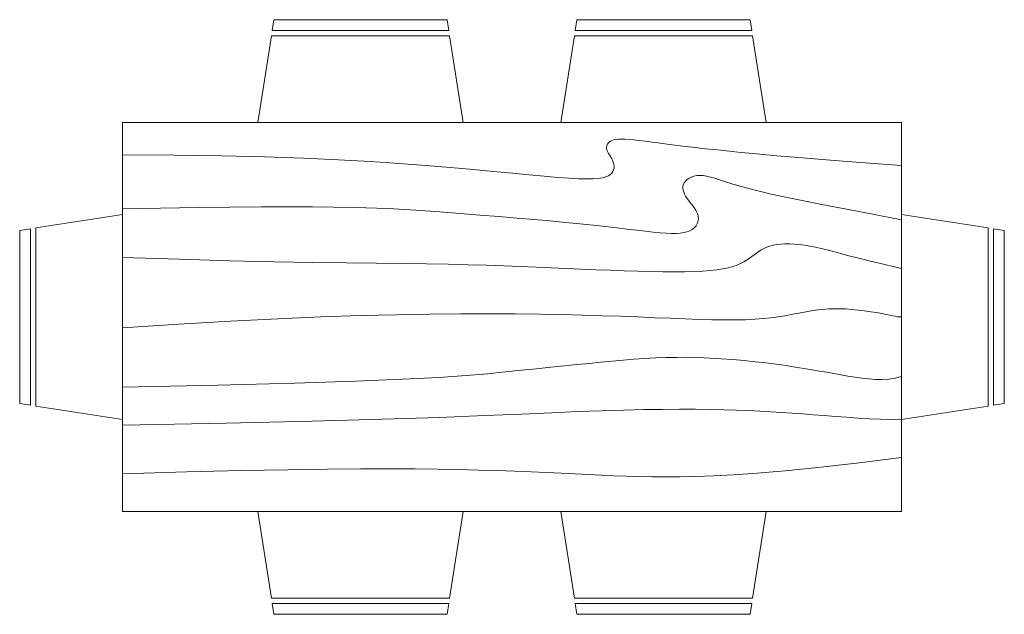
# Model space of a CAD drawing. Units: inches. Extents: x 2208 to 4689, y 1219 to 3512.
# Tile 5 of 5: x 4598 to 4689, y 3457 to 3512. Entities that reach past the tile are written whole.
import ezdxf

# ---------------------------------------------------------------- set-up
doc = ezdxf.new("R2010")
doc.units = ezdxf.units.IN
doc.layers.add('A-FURN', color=8, linetype='Continuous', lineweight=18)

# ---------------------------------------------------------------- blocks, each defined once
blk = doc.blocks.new('Dining Set - 36 x 72 in.')
for p, q in [((-22, 27.5), (-22.1562, 26.50042)), ((-22, 27.5), (-6, 27.5)), ((-5.8437, 26.49966), (-6, 27.5)), ((6, 27.5), (5.8438, 26.50042)), ((6, 27.5), (22, 27.5)), ((22.1563, 26.49966), (22, 27.5)), ((-5.8416, 26.5), (-22.1534, 26.5)), ((22.1584, 26.5), (5.8466, 26.5)), ((-22.2343, 26.00059), (-23.4847, 17.99762)), ((-22.2304, 26), (-5.7608, 26)), ((-4.5152, 17.99762), (-5.7655, 25.99926)), ((5.7657, 26.00059), (4.5153, 17.99762)), ((5.7696, 26), (22.2392, 26)), ((23.4848, 17.99762), (22.2345, 25.99926)), ((36, 18), (-36, 18)), ((-36, 18), (-36, -18)), ((36, -18), (36, 18)), ((-44.0006, 8.23428), (-35.9976, 9.48474)), ((44.0006, 8.23428), (35.9976, 9.48474)), ((-44, 8.23041), (-44, -8.23915)), ((44, 8.23041), (44, -8.23915)), ((-45.5, 8), (-44.5004, 8.15617)), ((-45.5, 8), (-45.5, -8)), ((-44.5, -8.15843), (-44.5, 8.15338)), ((44.5, -8.15843), (44.5, 8.15338)), ((45.5, 8), (44.5005, 8.15617)), ((45.5, 8), (45.5, -8)), ((-44.4997, -8.15631), (-45.5, -8)), ((44.4997, -8.15631), (45.5, -8)), ((-35.9976, -9.48476), (-43.9993, -8.2345)), ((35.9976, -9.48476), (43.9993, -8.2345)), ((-36, -18), (36, -18)), ((-22.2343, -26.0006), (-23.4847, -17.99762)), ((-4.5152, -17.99762), (-5.7655, -25.99928)), ((5.7657, -26.0006), (4.5153, -17.99762)), ((23.4848, -17.99762), (22.2345, -25.99928)), ((-22.2304, -26), (-5.7608, -26)), ((5.7696, -26), (22.2392, -26)), ((-22, -27.5), (-22.1562, -26.50044)), ((-5.8416, -26.5), (-22.1534, -26.5)), ((-5.8437, -26.49967), (-6, -27.5)), ((6, -27.5), (5.8438, -26.50044)), ((22.1584, -26.5), (5.8466, -26.5)), ((22.1563, -26.49967), (22, -27.5)), ((-22, -27.5), (-6, -27.5)), ((6, -27.5), (22, -27.5))]:
    blk.add_line(p, q)
for points in [[(-36, 15), (-31.1772, 14.97754), (-26.8079, 14.91406), (-22.8538, 14.81543), (-19.276, 14.6875), (-16.0362, 14.53613), (-13.0957, 14.36718), (-10.4159, 14.18652), (-7.9583, 14), (-5.6904, 13.81315), (-3.6035, 13.63021), (-1.6954, 13.45508), (0.0365, 13.29166), (1.5945, 13.14388), (2.9811, 13.01562), (4.1988, 12.9108), (5.25, 12.83333), (6.1393, 12.78613), (6.8802, 12.76823), (7.4883, 12.77767), (7.9792, 12.8125), (8.3685, 12.87077), (8.6719, 12.95052), (8.9049, 13.0498), (9.0833, 13.16666), (9.2205, 13.29899), (9.3216, 13.44401), (9.3895, 13.59879), (9.4271, 13.76041), (9.4373, 13.92594), (9.4232, 14.09245), (9.3875, 14.257), (9.3333, 14.41666), (9.2638, 14.56917), (9.1836, 14.71484), (9.0975, 14.85465), (9.0104, 14.98958), (8.9272, 15.1206), (8.8529, 15.2487), (8.7922, 15.37483), (8.75, 15.5), (8.7305, 15.62467), (8.7344, 15.74739), (8.7617, 15.86621), (8.8125, 15.97916), (8.8867, 16.08431), (8.9844, 16.17968), (9.1055, 16.26334), (9.25, 16.33333), (9.4189, 16.38802), (9.6172, 16.42708), (9.8506, 16.45052), (10.125, 16.45833), (10.4463, 16.45052), (10.8203, 16.42708), (11.2529, 16.38802), (11.75, 16.33333), (12.3184, 16.26318), (12.9694, 16.17838), (13.7151, 16.07991), (14.5677, 15.96875), (15.5395, 15.84586), (16.6426, 15.71224), (17.8893, 15.56884), (19.2917, 15.41666), (20.859, 15.25667), (22.5879, 15.08984), (24.4721, 14.91715), (26.5052, 14.73958), (28.6809, 14.5581), (30.9929, 14.3737), (33.4347, 14.18733), (36, 14)], [(-36, 10), (-28.9766, 10.14274), (-23.1725, 10.20442), (-18.4241, 10.19775), (-14.5677, 10.13541), (-11.4399, 10.03011), (-8.877, 9.89453), (-6.7154, 9.74137), (-4.7917, 9.58333), (-2.9698, 9.43082), (-1.2246, 9.28515), (0.4415, 9.14534), (2.026, 9.01041), (3.5266, 8.87939), (4.9408, 8.7513), (6.266, 8.62516), (7.5, 8.5), (8.6411, 8.37549), (9.6914, 8.2539), (10.6538, 8.13818), (11.5312, 8.03125), (12.3267, 7.93603), (13.043, 7.85547), (13.6831, 7.79248), (14.25, 7.75), (14.7471, 7.7303), (15.1797, 7.73307), (15.5537, 7.75732), (15.875, 7.80208), (16.1494, 7.86637), (16.3828, 7.94922), (16.5811, 8.04964), (16.75, 8.16666), (16.8944, 8.29915), (17.0143, 8.44531), (17.1089, 8.60319), (17.1771, 8.77083), (17.218, 8.94629), (17.2305, 9.1276), (17.2137, 9.31282), (17.1667, 9.5), (17.0895, 9.6875), (16.987, 9.875), (16.8649, 10.0625), (16.7292, 10.25), (16.5856, 10.4375), (16.4401, 10.625), (16.2985, 10.8125), (16.1667, 11), (16.05, 11.18733), (15.9518, 11.3737), (15.8752, 11.5581), (15.8229, 11.73958), (15.798, 11.91715), (15.8034, 12.08984), (15.842, 12.25667), (15.9167, 12.41666), (16.0295, 12.56836), (16.1784, 12.70833), (16.3605, 12.83268), (16.5729, 12.9375), (16.8127, 13.01888), (17.0768, 13.07291), (17.3625, 13.0957), (17.6667, 13.08333), (17.9894, 13.03312), (18.3418, 12.94726), (18.7382, 12.82918), (19.1927, 12.68229), (19.7195, 12.51001), (20.3327, 12.31575), (21.0465, 12.10294), (21.875, 11.875), (22.8357, 11.63354), (23.959, 11.37304), (25.2786, 11.08618), (26.8282, 10.76562), (28.6414, 10.40405), (30.752, 9.99414), (33.1936, 9.52856), (36, 9)], [(-36, 5.5), (-30.7157, 5.3348), (-26.069, 5.20963), (-21.9946, 5.11767), (-18.4271, 5.05208), (-15.3009, 5.00602), (-12.5508, 4.97265), (-10.1112, 4.94515), (-7.9167, 4.91666), (-5.909, 4.88167), (-4.0586, 4.83984), (-2.3429, 4.79215), (-0.7396, 4.73958), (0.7739, 4.6831), (2.22, 4.6237), (3.6213, 4.56233), (5, 4.5), (6.373, 4.43782), (7.7344, 4.3776), (9.0723, 4.32129), (10.375, 4.27083), (11.6309, 4.22819), (12.8281, 4.19531), (13.9551, 4.17415), (15, 4.16666), (15.954, 4.17448), (16.819, 4.19791), (17.6001, 4.23698), (18.3021, 4.29166), (18.9299, 4.36198), (19.4883, 4.44791), (19.9823, 4.54948), (20.4167, 4.66666), (20.7969, 4.79899), (21.1302, 4.94401), (21.4245, 5.09879), (21.6875, 5.26041), (21.9271, 5.42594), (22.1511, 5.59245), (22.3672, 5.757), (22.5834, 5.91666), (22.8065, 6.06868), (23.0404, 6.21093), (23.2879, 6.34147), (23.5521, 6.45833), (23.8358, 6.55957), (24.142, 6.64323), (24.4735, 6.70735), (24.8334, 6.75), (25.2235, 6.76969), (25.642, 6.76692), (26.0858, 6.74267), (26.5521, 6.69791), (27.0379, 6.63362), (27.5404, 6.55078), (28.0565, 6.45036), (28.5834, 6.33333), (29.1242, 6.19987), (29.7071, 6.04687), (30.3661, 5.87044), (31.1354, 5.66666), (32.0493, 5.43164), (33.142, 5.16146), (34.4475, 4.85221), (36, 4.5)], [(-36, -1), (-30.7915, -0.6591), (-26.0195, -0.38216), (-21.6519, -0.16284), (-17.6563, 0.00521), (-14.0005, 0.12833), (-10.6523, 0.21289), (-7.5796, 0.26522), (-4.75, 0.29166), (-2.134, 0.29793), (0.2878, 0.28711), (2.5317, 0.26163), (4.6146, 0.22396), (6.5529, 0.17651), (8.3633, 0.12174), (10.0623, 0.06209), (11.6667, 0), (13.1899, -0.06201), (14.6341, -0.1211), (15.9982, -0.17432), (17.2813, -0.21875), (18.4823, -0.25147), (19.6003, -0.26953), (20.6343, -0.27002), (21.5834, -0.25), (22.4481, -0.20768), (23.2357, -0.14584), (23.9549, -0.06836), (24.6146, 0.02083), (25.2235, 0.11784), (25.7904, 0.21875), (26.3241, 0.31966), (26.8334, 0.41666), (27.3265, 0.50618), (27.8099, 0.58593), (28.2894, 0.65397), (28.7709, 0.70833), (29.2601, 0.74707), (29.763, 0.76823), (30.2855, 0.76985), (30.8334, 0.75), (31.4088, 0.70784), (31.9994, 0.64713), (32.589, 0.57275), (33.1615, 0.48958), (33.7008, 0.4025), (34.1908, 0.3164), (34.6153, 0.23616), (34.9584, 0.16666), (35.2099, 0.11165), (35.3848, 0.07031), (35.504, 0.04069), (35.5886, 0.02083), (35.6594, 0.00879), (35.7377, 0.0026), (35.8442, 0.00032), (36, 0)], [(-36, -6.5), (-27.1843, -6.31267), (-20.084, -6.1263), (-14.469, -5.9419), (-10.1094, -5.76042), (-6.7752, -5.58285), (-4.2363, -5.41016), (-2.2629, -5.24333), (-0.625, -5.08334), (0.8708, -4.93099), (2.2715, -4.78646), (3.5872, -4.64974), (4.8281, -4.52084), (6.0046, -4.39974), (7.127, -4.28646), (8.2053, -4.18099), (9.25, -4.08334), (10.2705, -3.99382), (11.2734, -3.91407), (12.2647, -3.84603), (13.25, -3.79167), (14.2354, -3.75293), (15.2266, -3.73177), (16.2295, -3.73015), (17.25, -3.75), (18.2912, -3.79248), (19.3451, -3.85547), (20.4009, -3.93604), (21.4479, -4.03125), (22.4754, -4.13819), (23.4727, -4.25391), (24.4289, -4.37549), (25.3334, -4.5), (26.1785, -4.62492), (26.9694, -4.74935), (27.7145, -4.87281), (28.4219, -4.99479), (29.1, -5.11483), (29.7572, -5.23242), (30.4016, -5.34709), (31.0417, -5.45834), (31.6837, -5.56437), (32.3262, -5.65821), (32.9658, -5.73153), (33.599, -5.77604), (34.2224, -5.78345), (34.8327, -5.74545), (35.4264, -5.65373), (36, -5.5)], [(-36, -10), (-26.4022, -9.81299), (-18.4675, -9.62891), (-11.9839, -9.45069), (-6.7396, -9.28125), (-2.5226, -9.12354), (0.8789, -8.98047), (3.6769, -8.85498), (6.0833, -8.75), (8.2767, -8.66765), (10.3021, -8.60677), (12.1712, -8.56543), (13.8958, -8.54167), (15.4876, -8.53353), (16.9583, -8.53907), (18.3197, -8.55632), (19.5834, -8.58334), (20.7616, -8.61841), (21.8685, -8.66081), (22.9188, -8.71004), (23.9271, -8.76563), (24.9081, -8.82707), (25.8763, -8.89388), (26.8465, -8.96558), (27.8334, -9.04167), (28.8474, -9.12118), (29.8828, -9.20117), (30.93, -9.27824), (31.9792, -9.34896), (33.0205, -9.40991), (34.0443, -9.45768), (35.0407, -9.48885), (36, -9.5)], [(-36, -14.5), (-30.0881, -14.33513), (-25.0332, -14.21224), (-20.7312, -14.12647), (-17.0781, -14.07292), (-13.97, -14.04671), (-11.3027, -14.04297), (-8.9724, -14.05681), (-6.875, -14.08334), (-4.9224, -14.11833), (-3.0905, -14.16016), (-1.3709, -14.20785), (0.2448, -14.26042), (1.7647, -14.3169), (3.1973, -14.3763), (4.5507, -14.43767), (5.8333, -14.5), (7.0554, -14.5621), (8.235, -14.62175), (9.3922, -14.67652), (10.5469, -14.72396), (11.7192, -14.76164), (12.929, -14.78711), (14.1965, -14.79794), (15.5417, -14.79167), (16.9933, -14.76424), (18.6152, -14.70508), (20.4804, -14.60197), (22.6615, -14.44271), (25.2312, -14.21509), (28.2624, -13.9069), (31.8277, -13.50594), (36, -13)]]:
    blk.add_lwpolyline(points)

msp = doc.modelspace()

# ---------------------------------------------------------------- block references
at = {"layer": 'A-FURN'}
msp.add_blockref('Dining Set - 36 x 72 in.', (4643.4859, 3484.4591), dxfattribs=at)

doc.saveas('drawing.dxf')
